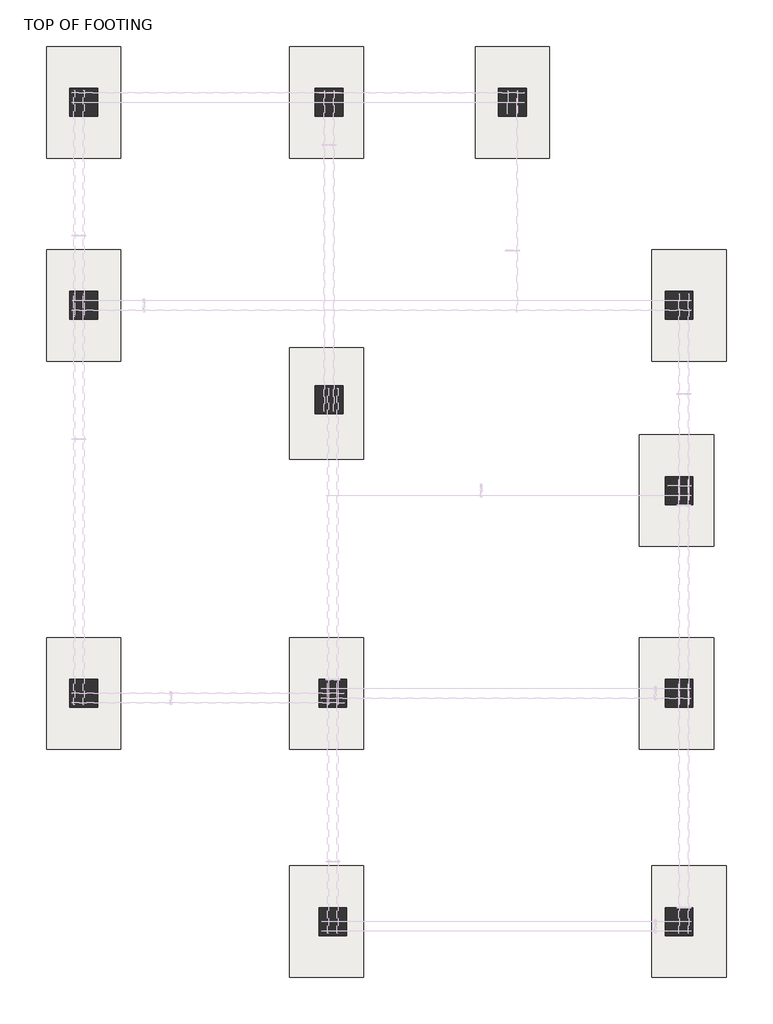
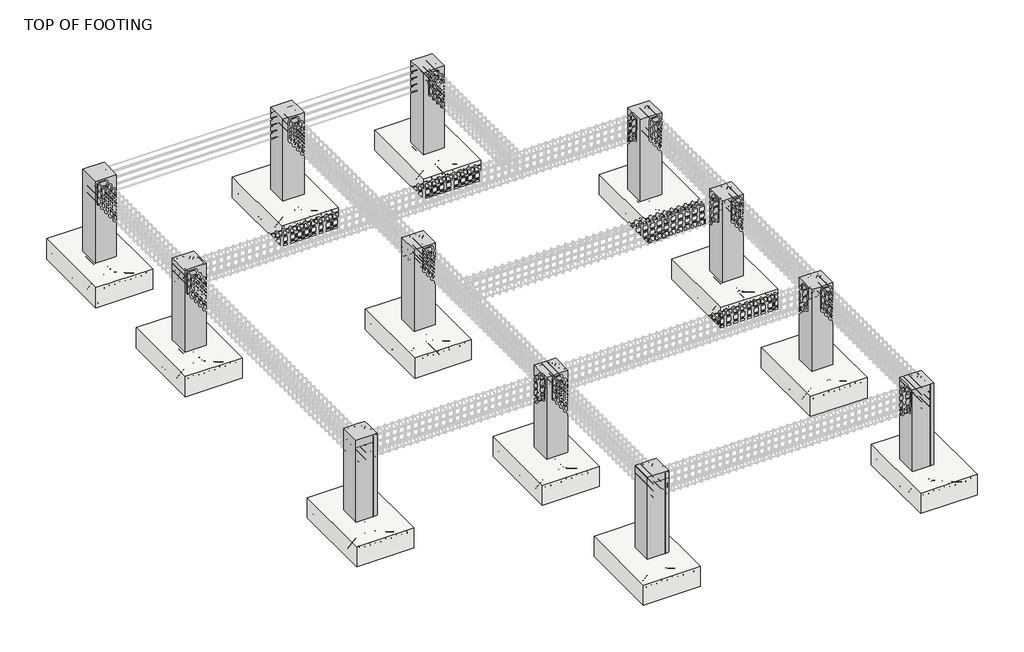
# One storey, part 1 of 11: 12 columns, 12 slabs.
"""IFC4 building model written with IfcOpenShell, lengths in millimetres."""

from ifc_helpers import new_model, si_unit, frame, origin, place, context, project, spatial, polyline, outline, extrude, faceted_brep, transform, mapped, element, save
from components import m_footing_rectangular_1800_x_1200_x_450mm_16ba7ea5

model = new_model("IFC4")

# Units and contexts
model_context = context("Model", 3, world=origin())
ifc_project = project(units=[si_unit("LENGTHUNIT", "METRE", prefix="MILLI")], contexts=[model_context])

# Site, building, storey
site = spatial("IfcSite", under=ifc_project)
building = spatial("IfcBuilding", under=site)
storey = spatial("IfcBuildingStorey", under=building, Name="TOP OF FOOTING", Elevation=-1828.8)

# Columns
placement = place(None, origin())
element("IfcColumn", 1, ObjectType="M_Concrete-Rectangular-Column", at=placement, inside=storey, context=model_context, shape_type="SweptSolid", body=[
    extrude(outline(polyline([(-6050.3728049, 6568.3757737), (-6050.3728049, 6118.3757737), (-6500.3728049, 6118.3757737), (-6500.3728049, 6568.3757737), (-6050.3728049, 6568.3757737)])), frame((0.0, 0.0, -1828.8), z_axis=(0.0, 0.0, 1.0), x_axis=(1.0, 0.0, 0.0)), (0.0, 0.0, 1.0), 1828.8),
])
element("IfcColumn", 2, ObjectType="M_Concrete-Rectangular-Column", at=placement, inside=storey, context=model_context, shape_type="Brep", body=[
    faceted_brep([(-2090.3728049, 6568.3757737, -1828.8), (-2090.3728049, 6118.3757737, -1828.8), (-2540.3728049, 6118.3757737, -1828.8), (-2540.3728049, 6568.3757737, -1828.8), (-2090.3728049, 6568.3757737, 0.0), (-2090.3728049, 6268.3757737, 0.0), (-2090.3728049, 6118.3757737, 0.0), (-2090.3728049, 6118.3757737, -300.0), (-2165.3728049, 6118.3757737, 0.0), (-2540.3728049, 6118.3757737, 0.0), (-2540.3728049, 6568.3757737, 0.0)], [[[0, 1, 2, 3]], [[1, 0, 4, 5, 6, 7]], [[2, 1, 7, 6, 8, 9]], [[3, 2, 9, 10]], [[0, 3, 10, 4]], [[10, 9, 8, 6, 5, 4]]]),
])
element("IfcColumn", 3, ObjectType="M_Concrete-Rectangular-Column", at=placement, inside=storey, context=model_context, shape_type="Brep", body=[
    faceted_brep([(869.6271951, 6568.3757737, -1828.8), (869.6271951, 6118.3757737, -1828.8), (419.6271951, 6118.3757737, -1828.8), (419.6271951, 6568.3757737, -1828.8), (869.6271951, 6568.3757737, 0.0), (869.6271951, 6118.3757737, 0.0), (494.6271951, 6118.3757737, 0.0), (419.6271951, 6118.3757737, 0.0), (419.6271951, 6118.3757737, -300.0), (419.6271951, 6268.3757737, 0.0), (419.6271951, 6568.3757737, 0.0)], [[[0, 1, 2, 3]], [[1, 0, 4, 5]], [[2, 1, 5, 6, 7, 8]], [[3, 2, 8, 7, 9, 10]], [[0, 3, 10, 4]], [[5, 4, 10, 9, 7, 6]]]),
])
element("IfcColumn", 4, ObjectType="M_Concrete-Rectangular-Column", at=placement, inside=storey, context=model_context, shape_type="Brep", body=[
    faceted_brep([(-6050.3728049, 3293.8544674, -1828.8), (-6050.3728049, 2843.8544674, -1828.8), (-6500.3728049, 2843.8544674, -1828.8), (-6500.3728049, 3293.8544674, -1828.8), (-6050.3728049, 3293.8544674, 0.0), (-6050.3728049, 2918.8544674, 0.0), (-6050.3728049, 2843.8544674, 0.0), (-6050.3728049, 2843.8544674, -300.0), (-6200.3728049, 2843.8544674, 0.0), (-6500.3728049, 2843.8544674, 0.0), (-6500.3728049, 3293.8544674, 0.0)], [[[0, 1, 2, 3]], [[1, 0, 4, 5, 6, 7]], [[2, 1, 7, 6, 8, 9]], [[3, 2, 9, 10]], [[0, 3, 10, 4]], [[10, 9, 8, 6, 5, 4]]]),
])
element("IfcColumn", 5, ObjectType="M_Concrete-Rectangular-Column", at=placement, inside=storey, context=model_context, shape_type="Brep", body=[
    faceted_brep([(-2090.3728049, 1770.6430781, -1828.8), (-2090.3728049, 1320.6430781, -1828.8), (-2540.3728049, 1320.6430781, -1828.8), (-2540.3728049, 1770.6430781, -1828.8), (-2090.3728049, 1770.6430781, -300.0), (-2090.3728049, 1770.6430781, 0.0), (-2090.3728049, 1320.6430781, 0.0), (-2090.3728049, 1320.6430781, -300.0), (-2105.3728049, 1320.6430781, 0.0), (-2405.3728049, 1320.6430781, 0.0), (-2540.3728049, 1320.6430781, 0.0), (-2540.3728049, 1320.6430781, -300.0), (-2540.3728049, 1770.6430781, 0.0), (-2540.3728049, 1770.6430781, -300.0), (-2465.3728049, 1770.6430781, 0.0), (-2165.3728049, 1770.6430781, 0.0)], [[[0, 1, 2, 3]], [[1, 0, 4, 5, 6, 7]], [[2, 1, 7, 6, 8, 9, 10, 11]], [[3, 2, 11, 10, 12, 13]], [[0, 3, 13, 12, 14, 15, 5, 4]], [[6, 5, 15, 14, 12, 10, 9, 8]]]),
])
element("IfcColumn", 6, ObjectType="M_Concrete-Rectangular-Column", at=placement, inside=storey, context=model_context, shape_type="Brep", body=[
    faceted_brep([(-6050.3728049, -2964.0513044, -1828.8), (-6050.3728049, -3414.0513044, -1828.8), (-6500.3728049, -3414.0513044, -1828.8), (-6500.3728049, -2964.0513044, -1828.8), (-6050.3728049, -2964.0513044, -300.0), (-6050.3728049, -2964.0513044, 0.0), (-6050.3728049, -3114.0513044, 0.0), (-6050.3728049, -3414.0513044, 0.0), (-6500.3728049, -3414.0513044, 0.0), (-6500.3728049, -2964.0513044, 0.0), (-6200.3728049, -2964.0513044, 0.0)], [[[0, 1, 2, 3]], [[1, 0, 4, 5, 6, 7]], [[2, 1, 7, 8]], [[3, 2, 8, 9]], [[0, 3, 9, 10, 5, 4]], [[8, 7, 6, 5, 10, 9]]]),
])
element("IfcColumn", 7, ObjectType="M_Concrete-Rectangular-Column", at=placement, inside=storey, context=model_context, shape_type="Brep", body=[
    faceted_brep([(-2030.3728049, -2964.0513044, -1828.8), (-2030.3728049, -3414.0513044, -1828.8), (-2480.3728049, -3414.0513044, -1828.8), (-2480.3728049, -2964.0513044, -1828.8), (-2030.3728049, -2964.0513044, -300.0), (-2030.3728049, -2964.0513044, 0.0), (-2030.3728049, -3039.0513044, 0.0), (-2030.3728049, -3339.0513044, 0.0), (-2030.3728049, -3414.0513044, 0.0), (-2030.3728049, -3414.0513044, -300.0), (-2105.3728049, -3414.0513044, 0.0), (-2480.3728049, -3414.0513044, 0.0), (-2480.3728049, -3114.0513044, 0.0), (-2480.3728049, -2964.0513044, 0.0), (-2480.3728049, -2964.0513044, -300.0), (-2405.3728049, -2964.0513044, 0.0), (-2105.3728049, -2964.0513044, 0.0)], [[[0, 1, 2, 3]], [[1, 0, 4, 5, 6, 7, 8, 9]], [[2, 1, 9, 8, 10, 11]], [[3, 2, 11, 12, 13, 14]], [[0, 3, 14, 13, 15, 16, 5, 4]], [[5, 16, 15, 13, 12, 11, 10, 8, 7, 6]]]),
])
element("IfcColumn", 8, ObjectType="M_Concrete-Rectangular-Column", at=placement, inside=storey, context=model_context, shape_type="Brep", body=[
    faceted_brep([(-2030.3728049, -6646.7750095, -1828.8), (-2030.3728049, -7096.7750095, -1828.8), (-2480.3728049, -7096.7750095, -1828.8), (-2480.3728049, -6646.7750095, -1828.8), (-2030.3728049, -6646.7750095, -300.0), (-2030.3728049, -6646.7750095, 0.0), (-2030.3728049, -6796.7750095, 0.0), (-2030.3728049, -7096.7750095, 0.0), (-2480.3728049, -7096.7750095, 0.0), (-2480.3728049, -6646.7750095, 0.0), (-2105.3728049, -6646.7750095, 0.0)], [[[0, 1, 2, 3]], [[1, 0, 4, 5, 6, 7]], [[2, 1, 7, 8]], [[3, 2, 8, 9]], [[0, 3, 9, 10, 5, 4]], [[8, 7, 6, 5, 10, 9]]]),
])
element("IfcColumn", 9, ObjectType="M_Concrete-Rectangular-Column", at=placement, inside=storey, context=model_context, shape_type="Brep", body=[
    faceted_brep([(3559.6271951, -6646.7750095, -1828.8), (3559.6271951, -7096.7750095, -1828.8), (3109.6271951, -7096.7750095, -1828.8), (3109.6271951, -6646.7750095, -1828.8), (3559.6271951, -6646.7750095, 0.0), (3559.6271951, -7096.7750095, 0.0), (3109.6271951, -7096.7750095, 0.0), (3109.6271951, -6796.7750095, 0.0), (3109.6271951, -6646.7750095, 0.0), (3109.6271951, -6646.7750095, -300.0), (3259.6271951, -6646.7750095, 0.0)], [[[0, 1, 2, 3]], [[1, 0, 4, 5]], [[2, 1, 5, 6]], [[3, 2, 6, 7, 8, 9]], [[0, 3, 9, 8, 10, 4]], [[5, 4, 10, 8, 7, 6]]]),
])
element("IfcColumn", 10, ObjectType="M_Concrete-Rectangular-Column", at=placement, inside=storey, context=model_context, shape_type="Brep", body=[
    faceted_brep([(3559.6271951, -2964.0513044, -1828.8), (3559.6271951, -3414.0513044, -1828.8), (3109.6271951, -3414.0513044, -1828.8), (3109.6271951, -2964.0513044, -1828.8), (3559.6271951, -2964.0513044, 0.0), (3559.6271951, -3414.0513044, 0.0), (3259.6271951, -3414.0513044, 0.0), (3109.6271951, -3414.0513044, 0.0), (3109.6271951, -3414.0513044, -300.0), (3109.6271951, -3339.0513044, 0.0), (3109.6271951, -3039.0513044, 0.0), (3109.6271951, -2964.0513044, 0.0), (3109.6271951, -2964.0513044, -300.0), (3259.6271951, -2964.0513044, 0.0)], [[[0, 1, 2, 3]], [[1, 0, 4, 5]], [[2, 1, 5, 6, 7, 8]], [[3, 2, 8, 7, 9, 10, 11, 12]], [[0, 3, 12, 11, 13, 4]], [[5, 4, 13, 11, 10, 9, 7, 6]]]),
])
element("IfcColumn", 11, ObjectType="M_Concrete-Rectangular-Column", at=placement, inside=storey, context=model_context, shape_type="Brep", body=[
    faceted_brep([(3559.6271951, 304.5469677, -1828.8), (3559.6271951, -145.4530323, -1828.8), (3109.6271951, -145.4530323, -1828.8), (3109.6271951, 304.5469677, -1828.8), (3559.6271951, 304.5469677, 0.0), (3559.6271951, -145.4530323, 0.0), (3259.6271951, -145.4530323, 0.0), (3109.6271951, -145.4530323, 0.0), (3109.6271951, -145.4530323, -300.0), (3109.6271951, -70.4530323, 0.0), (3109.6271951, 229.5469677, 0.0), (3109.6271951, 304.5469677, 0.0), (3109.6271951, 304.5469677, -300.0), (3259.6271951, 304.5469677, 0.0)], [[[0, 1, 2, 3]], [[1, 0, 4, 5]], [[2, 1, 5, 6, 7, 8]], [[3, 2, 8, 7, 9, 10, 11, 12]], [[0, 3, 12, 11, 13, 4]], [[5, 4, 13, 11, 10, 9, 7, 6]]]),
])
element("IfcColumn", 12, ObjectType="M_Concrete-Rectangular-Column", at=placement, inside=storey, context=model_context, shape_type="Brep", body=[
    faceted_brep([(3559.6271951, 3293.8544674, -1828.8), (3559.6271951, 2843.8544674, -1828.8), (3109.6271951, 2843.8544674, -1828.8), (3109.6271951, 3293.8544674, -1828.8), (3559.6271951, 3293.8544674, 0.0), (3559.6271951, 2843.8544674, 0.0), (3259.6271951, 2843.8544674, 0.0), (3109.6271951, 2843.8544674, 0.0), (3109.6271951, 2843.8544674, -300.0), (3109.6271951, 2918.8544674, 0.0), (3109.6271951, 3293.8544674, 0.0)], [[[0, 1, 2, 3]], [[1, 0, 4, 5]], [[2, 1, 5, 6, 7, 8]], [[3, 2, 8, 7, 9, 10]], [[0, 3, 10, 4]], [[5, 4, 10, 9, 7, 6]]]),
])

# Slabs
m_footing_rectangular_1800_x_1200_x_450mm_shape = m_footing_rectangular_1800_x_1200_x_450mm_16ba7ea5(model_context)
element("IfcSlab", 13, ObjectType="M_Footing-Rectangular : 1800 x 1200 x 450mm", at=placement, inside=storey, context=model_context, shape_type="MappedRepresentation", body=[
    mapped(m_footing_rectangular_1800_x_1200_x_450mm_shape, transform((-6275.3728049, 6343.3757737, -1828.8), x_axis=(1.0, 0.0, 0.0), y_axis=(0.0, 1.0, 0.0), z_axis=(0.0, 0.0, 1.0))),
])
element("IfcSlab", 14, ObjectType="M_Footing-Rectangular : 1800 x 1200 x 450mm", at=placement, inside=storey, context=model_context, shape_type="MappedRepresentation", body=[
    mapped(m_footing_rectangular_1800_x_1200_x_450mm_shape, transform((-2355.3728049, 6343.3757737, -1828.8), x_axis=(1.0, 0.0, 0.0), y_axis=(0.0, 1.0, 0.0), z_axis=(0.0, 0.0, 1.0))),
])
element("IfcSlab", 15, ObjectType="M_Footing-Rectangular : 1800 x 1200 x 450mm", at=placement, inside=storey, context=model_context, shape_type="MappedRepresentation", body=[
    mapped(m_footing_rectangular_1800_x_1200_x_450mm_shape, transform((644.6271951, 6343.3757737, -1828.8), x_axis=(1.0, 0.0, 0.0), y_axis=(0.0, 1.0, 0.0), z_axis=(0.0, 0.0, 1.0))),
])
element("IfcSlab", 16, ObjectType="M_Footing-Rectangular : 1800 x 1200 x 450mm", at=placement, inside=storey, context=model_context, shape_type="MappedRepresentation", body=[
    mapped(m_footing_rectangular_1800_x_1200_x_450mm_shape, transform((-6275.3728049, -3189.0513044, -1828.8), x_axis=(1.0, 0.0, 0.0), y_axis=(0.0, 1.0, 0.0), z_axis=(0.0, 0.0, 1.0))),
])
element("IfcSlab", 17, ObjectType="M_Footing-Rectangular : 1800 x 1200 x 450mm", at=placement, inside=storey, context=model_context, shape_type="MappedRepresentation", body=[
    mapped(m_footing_rectangular_1800_x_1200_x_450mm_shape, transform((-2355.3728049, -3189.0513044, -1828.8), x_axis=(1.0, 0.0, 0.0), y_axis=(0.0, 1.0, 0.0), z_axis=(0.0, 0.0, 1.0))),
])
element("IfcSlab", 18, ObjectType="M_Footing-Rectangular : 1800 x 1200 x 450mm", at=placement, inside=storey, context=model_context, shape_type="MappedRepresentation", body=[
    mapped(m_footing_rectangular_1800_x_1200_x_450mm_shape, transform((3294.6271951, -3189.0513044, -1828.8), x_axis=(1.0, 0.0, 0.0), y_axis=(0.0, 1.0, 0.0), z_axis=(0.0, 0.0, 1.0))),
])
element("IfcSlab", 19, ObjectType="M_Footing-Rectangular : 1800 x 1200 x 450mm", at=placement, inside=storey, context=model_context, shape_type="MappedRepresentation", body=[
    mapped(m_footing_rectangular_1800_x_1200_x_450mm_shape, transform((3494.6271951, -6871.7750095, -1828.8), x_axis=(1.0, 0.0, 0.0), y_axis=(0.0, 1.0, 0.0), z_axis=(0.0, 0.0, 1.0))),
])
element("IfcSlab", 20, ObjectType="M_Footing-Rectangular : 1800 x 1200 x 450mm", at=placement, inside=storey, context=model_context, shape_type="MappedRepresentation", body=[
    mapped(m_footing_rectangular_1800_x_1200_x_450mm_shape, transform((-6275.3728049, 3068.8544674, -1828.8), x_axis=(1.0, 0.0, 0.0), y_axis=(0.0, 1.0, 0.0), z_axis=(0.0, 0.0, 1.0))),
])
element("IfcSlab", 21, ObjectType="M_Footing-Rectangular : 1800 x 1200 x 450mm", at=placement, inside=storey, context=model_context, shape_type="MappedRepresentation", body=[
    mapped(m_footing_rectangular_1800_x_1200_x_450mm_shape, transform((-2355.3728049, 1485.6430781, -1828.8), x_axis=(1.0, 0.0, 0.0), y_axis=(0.0, 1.0, 0.0), z_axis=(0.0, 0.0, 1.0))),
])
element("IfcSlab", 22, ObjectType="M_Footing-Rectangular : 1800 x 1200 x 450mm", at=placement, inside=storey, context=model_context, shape_type="MappedRepresentation", body=[
    mapped(m_footing_rectangular_1800_x_1200_x_450mm_shape, transform((3494.6271951, 3068.8544674, -1828.8), x_axis=(1.0, 0.0, 0.0), y_axis=(0.0, 1.0, 0.0), z_axis=(0.0, 0.0, 1.0))),
])
element("IfcSlab", 23, ObjectType="M_Footing-Rectangular : 1800 x 1200 x 450mm", at=placement, inside=storey, context=model_context, shape_type="MappedRepresentation", body=[
    mapped(m_footing_rectangular_1800_x_1200_x_450mm_shape, transform((3294.6271951, 79.5469677, -1828.8), x_axis=(1.0, 0.0, 0.0), y_axis=(0.0, 1.0, 0.0), z_axis=(0.0, 0.0, 1.0))),
])
element("IfcSlab", 24, ObjectType="M_Footing-Rectangular : 1800 x 1200 x 450mm", at=placement, inside=storey, context=model_context, shape_type="MappedRepresentation", body=[
    mapped(m_footing_rectangular_1800_x_1200_x_450mm_shape, transform((-2355.3728049, -6871.7750095, -1828.8), x_axis=(1.0, 0.0, 0.0), y_axis=(0.0, 1.0, 0.0), z_axis=(0.0, 0.0, 1.0))),
])

save(model, "model.ifc")

# Revit data of these elements
# Grids (mm)
#   "1": line (-6275.373, -14115.179) -> (-6275.373, 22134.037)
#   "2": line (-2355.373, -14115.179) -> (-2355.373, 22134.037)
#   "3": line (644.627, -14115.179) -> (644.627, 22134.037)
#   "4": line (3494.627, -14115.179) -> (3494.627, 22134.037)
#   "A": line (8130.772, 6343.376) -> (-11004.216, 6343.376)
#   "B": line (8130.772, 3068.854) -> (-10256.17, 3068.854)
#   "C": line (8130.772, 1485.643) -> (-10527.87, 1485.643)
#   "D": line (8130.772, 79.547) -> (-11076.18, 79.547)
#   "E": line (8130.772, -3189.051) -> (-11076.18, -3189.051)
#   "F": line (8130.772, -6871.775) -> (-11076.18, -6871.775)
# Type "M_Concrete-Rectangular-Column"
#   b = 450 mm
#   h = 450 mm
#   Structural Material [instance default] = Concrete, Cast-in-Place gray
# Type "M_Footing-Rectangular : 1800 x 1200 x 450mm"
#   Width = 1200 mm
#   Length = 1800 mm
#   Foundation Thickness = 450 mm
#   Structural Material [instance default] = Concrete, Cast-in-Place gray
#   Assembly Code = ""
# Elements 1, 2, 3, 4, 5, 6, 7, 8, 9, 10, 11, 12 (IfcColumn, "M_Concrete-Rectangular-Column")
#   Structural Material = Concrete, Cast-in-Place gray
#   Phase Created = New Construction
#   Materials on its faces: "Concrete, Cast-in-Place gray"
# Elements 13, 14, 15, 16, 17, 18, 19, 20, 21, 22, 23, 24 (IfcSlab, "M_Footing-Rectangular : 1800 x 1200 x 450mm")
#   Structural Material = Concrete, Cast-in-Place gray
#   Phase Created = New Construction
#   Materials on its faces: "Concrete, Cast-in-Place gray"
# Materials
#   "Concrete, Cast-in-Place gray": class "Concrete", colour RGB 192 192 192, transparency 0, Description = "Cast-in-place concrete", Cost = 0
